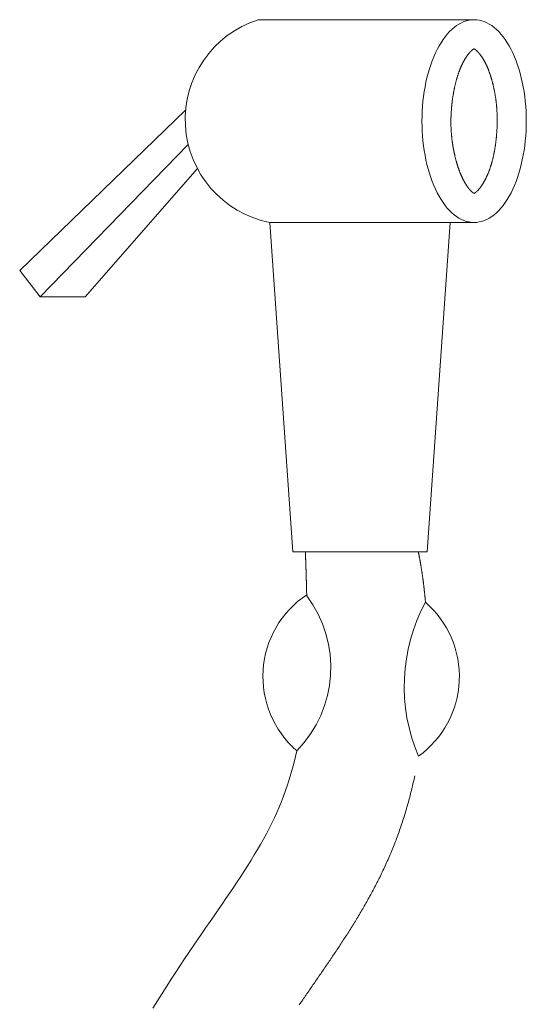
# Model space of a CAD drawing. Units: inches. Extents: x 64 to 1167, y 117 to 939.
# Tile 32 of 56: x 1044.798 to 1047.594, y 453.834 to 459.271. Entities that reach past the tile are written whole.
import ezdxf

# ---------------------------------------------------------------- set-up
doc = ezdxf.new("R2010")
doc.units = ezdxf.units.IN
doc.header["$MEASUREMENT"] = 0
doc.layers.add('A-FLOR-FIXT', color=8, linetype='Continuous', lineweight=18)

# ---------------------------------------------------------------- blocks, each defined once
blk = doc.blocks.new('A$C01277C2D')
for p, q in [((2.2872, 12.2015), (1.3927, 12.2015)), ((1.0923, 11.8276), (0.4045, 11.1621)), ((0.489, 11.0535), (1.103, 11.6838)), ((0.6759, 11.0535), (1.1406, 11.5847)), ((2.2872, 11.3612), (1.4404, 11.3612)), ((1.4404, 11.3612), (1.5365, 9.996)), ((2.0923, 9.996), (2.1874, 11.3612)), ((0.4045, 11.1621), (0.489, 11.0535)), ((0.489, 11.0535), (0.6759, 11.0535)), ((1.5365, 9.996), (2.0923, 9.996))]:
    blk.add_line(p, q)
for points in [[(2.2872, 12.2015, 0), (2.2766, 12.201, 0), (2.266, 12.1995, 0), (2.2555, 12.197, 0), (2.245, 12.1935, 0), (2.2347, 12.1889, 0), (2.2245, 12.1834, 0), (2.2144, 12.177, 0), (2.2045, 12.1695, 0), (2.1948, 12.1612, 0), (2.1853, 12.1519, 0), (2.1761, 12.1418, 0), (2.1671, 12.1307, 0), (2.1585, 12.1188, 0), (2.1501, 12.1062, 0), (2.1421, 12.0927, 0), (2.1344, 12.0785, 0), (2.1271, 12.0635, 0), (2.1201, 12.0479, 0), (2.1136, 12.0317, 0), (2.1075, 12.0148, 0), (2.1018, 11.9974, 0), (2.0966, 11.9794, 0), (2.0918, 11.961, 0), (2.0875, 11.9422, 0), (2.0837, 11.9229, 0), (2.0804, 11.9033, 0), (2.0776, 11.8835, 0), (2.0752, 11.8633, 0), (2.0734, 11.843, 0), (2.0721, 11.8226, 0), (2.0713, 11.802, 0), (2.0711, 11.7814, 0), (2.0713, 11.7608, 0), (2.0721, 11.7402, 0), (2.0734, 11.7197, 0), (2.0752, 11.6994, 0), (2.0776, 11.6793, 0), (2.0804, 11.6594, 0), (2.0837, 11.6398, 0), (2.0875, 11.6206, 0), (2.0918, 11.6017, 0), (2.0966, 11.5833, 0), (2.1018, 11.5654, 0), (2.1075, 11.548, 0), (2.1136, 11.5311, 0), (2.1201, 11.5148, 0), (2.1271, 11.4992, 0), (2.1344, 11.4843, 0), (2.1421, 11.4701, 0), (2.1501, 11.4566, 0), (2.1585, 11.4439, 0), (2.1671, 11.432, 0), (2.1761, 11.421, 0), (2.1853, 11.4108, 0), (2.1948, 11.4016, 0), (2.2045, 11.3932, 0), (2.2144, 11.3858, 0), (2.2245, 11.3793, 0), (2.2347, 11.3738, 0), (2.245, 11.3693, 0), (2.2555, 11.3658, 0), (2.266, 11.3633, 0), (2.2766, 11.3617, 0), (2.2872, 11.3612, 0), (2.2978, 11.3617, 0), (2.3084, 11.3633, 0), (2.3189, 11.3658, 0), (2.3294, 11.3693, 0), (2.3397, 11.3738, 0), (2.35, 11.3793, 0), (2.36, 11.3858, 0), (2.3699, 11.3932, 0), (2.3796, 11.4016, 0), (2.3891, 11.4108, 0), (2.3983, 11.421, 0), (2.4073, 11.432, 0), (2.416, 11.4439, 0), (2.4243, 11.4566, 0), (2.4324, 11.4701, 0), (2.44, 11.4843, 0), (2.4474, 11.4992, 0), (2.4543, 11.5148, 0), (2.4608, 11.5311, 0), (2.4669, 11.548, 0), (2.4726, 11.5654, 0), (2.4778, 11.5833, 0), (2.4826, 11.6017, 0), (2.4869, 11.6206, 0), (2.4907, 11.6398, 0), (2.494, 11.6594, 0), (2.4969, 11.6793, 0), (2.4992, 11.6994, 0), (2.501, 11.7197, 0), (2.5023, 11.7402, 0), (2.5031, 11.7608, 0), (2.5034, 11.7814, 0), (2.5031, 11.802, 0), (2.5023, 11.8226, 0), (2.501, 11.843, 0), (2.4992, 11.8633, 0), (2.4969, 11.8835, 0), (2.494, 11.9033, 0), (2.4907, 11.9229, 0), (2.4869, 11.9422, 0), (2.4826, 11.961, 0), (2.4778, 11.9794, 0), (2.4726, 11.9974, 0), (2.4669, 12.0148, 0), (2.4608, 12.0317, 0), (2.4543, 12.0479, 0), (2.4474, 12.0635, 0), (2.44, 12.0785, 0), (2.4324, 12.0927, 0), (2.4243, 12.1062, 0), (2.416, 12.1188, 0), (2.4073, 12.1307, 0), (2.3983, 12.1418, 0), (2.3891, 12.1519, 0), (2.3796, 12.1612, 0), (2.3699, 12.1695, 0), (2.36, 12.177, 0), (2.35, 12.1834, 0), (2.3397, 12.1889, 0), (2.3294, 12.1935, 0), (2.3189, 12.197, 0), (2.3084, 12.1995, 0), (2.2978, 12.201, 0), (2.2872, 12.2015, 0)], [(2.2871, 12.0812, 0), (2.2869, 12.0811, 0), (2.2868, 12.081, 0), (2.2866, 12.0809, 0), (2.2864, 12.0808, 0), (2.2861, 12.0807, 0), (2.2859, 12.0805, 0), (2.2857, 12.0804, 0), (2.2854, 12.0802, 0), (2.2851, 12.08, 0), (2.2849, 12.0799, 0), (2.2846, 12.0797, 0), (2.2843, 12.0795, 0), (2.284, 12.0793, 0), (2.2836, 12.079, 0), (2.2833, 12.0788, 0), (2.283, 12.0785, 0), (2.2826, 12.0783, 0), (2.2822, 12.078, 0), (2.2819, 12.0777, 0), (2.2815, 12.0774, 0), (2.2811, 12.0771, 0), (2.2807, 12.0768, 0), (2.2803, 12.0765, 0), (2.2799, 12.0761, 0), (2.2794, 12.0758, 0), (2.279, 12.0754, 0), (2.2786, 12.075, 0), (2.2781, 12.0746, 0), (2.2776, 12.0742, 0), (2.2772, 12.0738, 0), (2.2767, 12.0734, 0), (2.2762, 12.073, 0), (2.2757, 12.0725, 0), (2.2752, 12.072, 0), (2.2747, 12.0715, 0), (2.2742, 12.071, 0), (2.2737, 12.0705, 0), (2.2731, 12.07, 0), (2.2726, 12.0695, 0), (2.2721, 12.0689, 0), (2.2715, 12.0684, 0), (2.271, 12.0678, 0), (2.2704, 12.0672, 0), (2.2698, 12.0666, 0), (2.2693, 12.0659, 0), (2.2687, 12.0653, 0), (2.2681, 12.0647, 0), (2.2675, 12.064, 0), (2.267, 12.0633, 0), (2.2664, 12.0626, 0), (2.2658, 12.0619, 0), (2.2652, 12.0612, 0), (2.2645, 12.0604, 0), (2.2639, 12.0597, 0), (2.2633, 12.0589, 0), (2.2627, 12.0581, 0), (2.2621, 12.0573, 0), (2.2615, 12.0565, 0), (2.2608, 12.0557, 0), (2.2602, 12.0548, 0), (2.2596, 12.054, 0), (2.2589, 12.0531, 0), (2.2583, 12.0522, 0), (2.2577, 12.0513, 0), (2.257, 12.0504, 0), (2.2564, 12.0494, 0), (2.2557, 12.0485, 0), (2.2551, 12.0475, 0), (2.2545, 12.0466, 0), (2.2538, 12.0456, 0), (2.2532, 12.0446, 0), (2.2525, 12.0436, 0), (2.2519, 12.0426, 0), (2.2512, 12.0415, 0), (2.2506, 12.0405, 0), (2.25, 12.0394, 0), (2.2493, 12.0384, 0), (2.2487, 12.0373, 0), (2.248, 12.0362, 0), (2.2474, 12.0351, 0), (2.2467, 12.0339, 0), (2.2461, 12.0328, 0), (2.2454, 12.0317, 0), (2.2448, 12.0305, 0), (2.2441, 12.0293, 0), (2.2435, 12.0281, 0), (2.2428, 12.0269, 0), (2.2422, 12.0257, 0), (2.2416, 12.0245, 0), (2.2409, 12.0232, 0), (2.2403, 12.022, 0), (2.2396, 12.0207, 0), (2.239, 12.0195, 0), (2.2384, 12.0182, 0), (2.2377, 12.0169, 0), (2.2371, 12.0155, 0), (2.2365, 12.0142, 0), (2.2358, 12.0129, 0), (2.2352, 12.0115, 0), (2.2346, 12.0102, 0), (2.234, 12.0088, 0), (2.2333, 12.0074, 0), (2.2327, 12.006, 0), (2.2321, 12.0046, 0), (2.2315, 12.0032, 0), (2.2309, 12.0017, 0), (2.2303, 12.0003, 0), (2.2297, 11.9988, 0), (2.2291, 11.9974, 0), (2.2285, 11.9959, 0), (2.2279, 11.9944, 0), (2.2273, 11.9929, 0), (2.2267, 11.9913, 0), (2.2261, 11.9898, 0), (2.2255, 11.9883, 0), (2.225, 11.9867, 0), (2.2244, 11.9851, 0), (2.2238, 11.9836, 0), (2.2233, 11.982, 0), (2.2227, 11.9804, 0), (2.2221, 11.9788, 0), (2.2216, 11.9771, 0), (2.221, 11.9755, 0), (2.2205, 11.9739, 0), (2.22, 11.9722, 0), (2.2194, 11.9706, 0), (2.2189, 11.9689, 0), (2.2184, 11.9672, 0), (2.2178, 11.9655, 0), (2.2173, 11.9638, 0), (2.2168, 11.9621, 0), (2.2163, 11.9604, 0), (2.2158, 11.9586, 0), (2.2153, 11.9569, 0), (2.2148, 11.9551, 0), (2.2143, 11.9534, 0), (2.2138, 11.9516, 0), (2.2133, 11.9498, 0), (2.2128, 11.948, 0), (2.2123, 11.9462, 0), (2.2119, 11.9444, 0), (2.2114, 11.9426, 0), (2.2109, 11.9408, 0), (2.2105, 11.939, 0), (2.21, 11.9371, 0), (2.2096, 11.9353, 0), (2.2091, 11.9334, 0), (2.2087, 11.9316, 0), (2.2082, 11.9297, 0), (2.2078, 11.9278, 0), (2.2074, 11.9259, 0), (2.2069, 11.924, 0), (2.2065, 11.9221, 0), (2.2061, 11.9202, 0), (2.2057, 11.9183, 0), (2.2053, 11.9164, 0), (2.2049, 11.9145, 0), (2.2045, 11.9125, 0), (2.2041, 11.9106, 0), (2.2037, 11.9087, 0), (2.2034, 11.9067, 0), (2.203, 11.9047, 0), (2.2026, 11.9028, 0), (2.2023, 11.9008, 0), (2.2019, 11.8988, 0), (2.2016, 11.8968, 0), (2.2012, 11.8949, 0), (2.2009, 11.8929, 0), (2.2005, 11.8909, 0), (2.2002, 11.8889, 0), (2.1999, 11.8868, 0), (2.1996, 11.8848, 0), (2.1992, 11.8828, 0), (2.1989, 11.8808, 0), (2.1986, 11.8788, 0), (2.1983, 11.8767, 0), (2.198, 11.8747, 0), (2.1978, 11.8726, 0), (2.1975, 11.8706, 0), (2.1972, 11.8685, 0), (2.1969, 11.8665, 0), (2.1967, 11.8644, 0), (2.1964, 11.8623, 0), (2.1961, 11.8603, 0), (2.1959, 11.8582, 0), (2.1957, 11.8561, 0), (2.1954, 11.854, 0), (2.1952, 11.852, 0), (2.195, 11.8499, 0), (2.1947, 11.8478, 0), (2.1945, 11.8457, 0), (2.1943, 11.8436, 0), (2.1941, 11.8415, 0), (2.1939, 11.8394, 0), (2.1938, 11.8373, 0), (2.1936, 11.8352, 0), (2.1934, 11.8331, 0), (2.1932, 11.831, 0), (2.1931, 11.8289, 0), (2.1929, 11.8268, 0), (2.1928, 11.8246, 0), (2.1926, 11.8225, 0), (2.1925, 11.8204, 0), (2.1923, 11.8183, 0), (2.1922, 11.8162, 0), (2.1921, 11.814, 0), (2.192, 11.8119, 0), (2.1919, 11.8098, 0), (2.1918, 11.8077, 0), (2.1917, 11.8055, 0), (2.1916, 11.8034, 0), (2.1915, 11.8013, 0), (2.1915, 11.7992, 0), (2.1914, 11.797, 0), (2.1913, 11.7949, 0), (2.1913, 11.7928, 0), (2.1912, 11.7906, 0), (2.1912, 11.7885, 0), (2.1912, 11.7864, 0), (2.1911, 11.7842, 0), (2.1911, 11.7821, 0), (2.1911, 11.78, 0), (2.1911, 11.7779, 0), (2.1911, 11.7757, 0), (2.1911, 11.7736, 0), (2.1911, 11.7715, 0), (2.1912, 11.7694, 0), (2.1912, 11.7672, 0), (2.1912, 11.7651, 0), (2.1913, 11.763, 0), (2.1913, 11.7609, 0), (2.1914, 11.7588, 0), (2.1915, 11.7566, 0), (2.1915, 11.7545, 0), (2.1916, 11.7524, 0), (2.1917, 11.7503, 0), (2.1918, 11.7482, 0), (2.1919, 11.7461, 0), (2.192, 11.744, 0), (2.1922, 11.7419, 0), (2.1923, 11.7398, 0), (2.1924, 11.7376, 0), (2.1926, 11.7355, 0), (2.1927, 11.7335, 0), (2.1929, 11.7314, 0), (2.193, 11.7293, 0), (2.1932, 11.7272, 0), (2.1934, 11.7251, 0), (2.1936, 11.723, 0), (2.1938, 11.7209, 0), (2.194, 11.7188, 0), (2.1942, 11.7168, 0), (2.1944, 11.7147, 0), (2.1946, 11.7126, 0), (2.1948, 11.7106, 0), (2.1951, 11.7085, 0), (2.1953, 11.7064, 0), (2.1955, 11.7044, 0), (2.1958, 11.7023, 0), (2.1961, 11.7003, 0), (2.1963, 11.6982, 0), (2.1966, 11.6962, 0), (2.1969, 11.6941, 0), (2.1972, 11.6921, 0), (2.1974, 11.6901, 0), (2.1977, 11.6881, 0), (2.198, 11.686, 0), (2.1984, 11.684, 0), (2.1987, 11.682, 0), (2.199, 11.68, 0), (2.1993, 11.678, 0), (2.1996, 11.676, 0), (2.2, 11.674, 0), (2.2003, 11.672, 0), (2.2007, 11.67, 0), (2.201, 11.6681, 0), (2.2014, 11.6661, 0), (2.2018, 11.6641, 0), (2.2021, 11.6622, 0), (2.2025, 11.6602, 0), (2.2029, 11.6583, 0), (2.2033, 11.6563, 0), (2.2037, 11.6544, 0), (2.2041, 11.6525, 0), (2.2045, 11.6505, 0), (2.2049, 11.6486, 0), (2.2053, 11.6467, 0), (2.2057, 11.6448, 0), (2.2061, 11.6429, 0), (2.2066, 11.641, 0), (2.207, 11.6391, 0), (2.2074, 11.6372, 0), (2.2079, 11.6354, 0), (2.2083, 11.6335, 0), (2.2088, 11.6316, 0), (2.2092, 11.6298, 0), (2.2097, 11.6279, 0), (2.2102, 11.6261, 0), (2.2106, 11.6243, 0), (2.2111, 11.6224, 0), (2.2116, 11.6206, 0), (2.2121, 11.6188, 0), (2.2126, 11.617, 0), (2.2131, 11.6152, 0), (2.2136, 11.6135, 0), (2.2141, 11.6117, 0), (2.2146, 11.6099, 0), (2.2151, 11.6081, 0), (2.2156, 11.6064, 0), (2.2161, 11.6047, 0), (2.2166, 11.6029, 0), (2.2172, 11.6012, 0), (2.2177, 11.5995, 0), (2.2182, 11.5978, 0), (2.2188, 11.5961, 0), (2.2193, 11.5944, 0), (2.2199, 11.5927, 0), (2.2204, 11.591, 0), (2.221, 11.5894, 0), (2.2215, 11.5877, 0), (2.2221, 11.5861, 0), (2.2226, 11.5844, 0), (2.2232, 11.5828, 0), (2.2238, 11.5812, 0), (2.2243, 11.5796, 0), (2.2249, 11.578, 0), (2.2255, 11.5764, 0), (2.2261, 11.5749, 0), (2.2267, 11.5733, 0), (2.2273, 11.5717, 0), (2.2279, 11.5702, 0), (2.2285, 11.5687, 0), (2.2291, 11.5671, 0), (2.2297, 11.5656, 0), (2.2303, 11.5641, 0), (2.2309, 11.5626, 0), (2.2315, 11.5612, 0), (2.2321, 11.5597, 0), (2.2327, 11.5582, 0), (2.2333, 11.5568, 0), (2.234, 11.5554, 0), (2.2346, 11.554, 0), (2.2352, 11.5526, 0), (2.2358, 11.5512, 0), (2.2365, 11.5498, 0), (2.2371, 11.5485, 0), (2.2377, 11.5471, 0), (2.2384, 11.5458, 0), (2.239, 11.5445, 0), (2.2396, 11.5432, 0), (2.2403, 11.5419, 0), (2.2409, 11.5406, 0), (2.2416, 11.5394, 0), (2.2422, 11.5381, 0), (2.2428, 11.5369, 0), (2.2435, 11.5357, 0), (2.2441, 11.5345, 0), (2.2448, 11.5333, 0), (2.2454, 11.5321, 0), (2.246, 11.531, 0), (2.2467, 11.5298, 0), (2.2473, 11.5287, 0), (2.248, 11.5276, 0), (2.2486, 11.5265, 0), (2.2493, 11.5254, 0), (2.2499, 11.5243, 0), (2.2505, 11.5233, 0), (2.2512, 11.5222, 0), (2.2518, 11.5212, 0), (2.2525, 11.5202, 0), (2.2531, 11.5191, 0), (2.2537, 11.5182, 0), (2.2544, 11.5172, 0), (2.255, 11.5162, 0), (2.2556, 11.5153, 0), (2.2562, 11.5143, 0), (2.2569, 11.5134, 0), (2.2575, 11.5125, 0), (2.2581, 11.5116, 0), (2.2587, 11.5107, 0), (2.2593, 11.5098, 0), (2.2599, 11.509, 0), (2.2605, 11.5081, 0), (2.2612, 11.5073, 0), (2.2618, 11.5065, 0), (2.2624, 11.5057, 0), (2.2629, 11.5049, 0), (2.2635, 11.5041, 0), (2.2641, 11.5034, 0), (2.2647, 11.5026, 0), (2.2653, 11.5019, 0), (2.2659, 11.5012, 0), (2.2664, 11.5005, 0), (2.267, 11.4998, 0), (2.2676, 11.4991, 0), (2.2681, 11.4985, 0), (2.2687, 11.4978, 0), (2.2692, 11.4972, 0), (2.2698, 11.4966, 0), (2.2703, 11.4959, 0), (2.2708, 11.4953, 0), (2.2714, 11.4948, 0), (2.2719, 11.4942, 0), (2.2724, 11.4936, 0), (2.2729, 11.4931, 0), (2.2734, 11.4926, 0), (2.2739, 11.4921, 0), (2.2744, 11.4916, 0), (2.2749, 11.4911, 0), (2.2754, 11.4906, 0), (2.2759, 11.4901, 0), (2.2763, 11.4897, 0), (2.2768, 11.4892, 0), (2.2772, 11.4888, 0), (2.2777, 11.4884, 0), (2.2781, 11.488, 0), (2.2786, 11.4876, 0), (2.279, 11.4873, 0), (2.2794, 11.4869, 0), (2.2798, 11.4866, 0), (2.2802, 11.4863, 0), (2.2806, 11.4859, 0), (2.281, 11.4856, 0), (2.2814, 11.4854, 0), (2.2817, 11.4851, 0), (2.2821, 11.4848, 0), (2.2825, 11.4846, 0), (2.2828, 11.4843, 0), (2.2831, 11.4841, 0), (2.2835, 11.4839, 0), (2.2838, 11.4837, 0), (2.2841, 11.4835, 0), (2.2844, 11.4833, 0), (2.2847, 11.4831, 0), (2.285, 11.4829, 0), (2.2852, 11.4828, 0), (2.2855, 11.4826, 0), (2.2858, 11.4825, 0), (2.286, 11.4823, 0), (2.2862, 11.4822, 0), (2.2865, 11.4821, 0), (2.2867, 11.482, 0), (2.2869, 11.4818, 0), (2.2871, 11.4818, 0), (2.2873, 11.4817, 0), (2.2875, 11.4816, 0), (2.2876, 11.4815, 0)], [(2.2876, 11.4815, 0), (2.2878, 11.4816, 0), (2.2881, 11.4817, 0), (2.2883, 11.4819, 0), (2.2886, 11.482, 0), (2.2888, 11.4822, 0), (2.2891, 11.4824, 0), (2.2894, 11.4826, 0), (2.2898, 11.4828, 0), (2.2901, 11.4831, 0), (2.2904, 11.4833, 0), (2.2908, 11.4836, 0), (2.2912, 11.4838, 0), (2.2916, 11.4841, 0), (2.292, 11.4845, 0), (2.2924, 11.4848, 0), (2.2929, 11.4851, 0), (2.2933, 11.4855, 0), (2.2938, 11.4859, 0), (2.2943, 11.4863, 0), (2.2948, 11.4867, 0), (2.2953, 11.4871, 0), (2.2958, 11.4875, 0), (2.2963, 11.488, 0), (2.2969, 11.4885, 0), (2.2974, 11.489, 0), (2.298, 11.4895, 0), (2.2985, 11.49, 0), (2.2991, 11.4906, 0), (2.2997, 11.4911, 0), (2.3003, 11.4917, 0), (2.3009, 11.4923, 0), (2.3015, 11.493, 0), (2.3021, 11.4936, 0), (2.3028, 11.4943, 0), (2.3034, 11.4949, 0), (2.3041, 11.4956, 0), (2.3047, 11.4963, 0), (2.3054, 11.4971, 0), (2.306, 11.4978, 0), (2.3067, 11.4986, 0), (2.3074, 11.4994, 0), (2.3081, 11.5002, 0), (2.3088, 11.501, 0), (2.3095, 11.5019, 0), (2.3102, 11.5027, 0), (2.3109, 11.5036, 0), (2.3116, 11.5045, 0), (2.3123, 11.5055, 0), (2.313, 11.5064, 0), (2.3138, 11.5074, 0), (2.3145, 11.5084, 0), (2.3152, 11.5094, 0), (2.3159, 11.5104, 0), (2.3167, 11.5115, 0), (2.3174, 11.5125, 0), (2.3181, 11.5136, 0), (2.3189, 11.5147, 0), (2.3196, 11.5159, 0), (2.3204, 11.517, 0), (2.3211, 11.5182, 0), (2.3219, 11.5193, 0), (2.3226, 11.5205, 0), (2.3234, 11.5218, 0), (2.3241, 11.523, 0), (2.3249, 11.5243, 0), (2.3256, 11.5255, 0), (2.3264, 11.5268, 0), (2.3271, 11.5281, 0), (2.3279, 11.5294, 0), (2.3287, 11.5308, 0), (2.3294, 11.5321, 0), (2.3302, 11.5335, 0), (2.3309, 11.5349, 0), (2.3317, 11.5363, 0), (2.3324, 11.5377, 0), (2.3332, 11.5392, 0), (2.3339, 11.5406, 0), (2.3347, 11.5421, 0), (2.3354, 11.5436, 0), (2.3362, 11.5451, 0), (2.3369, 11.5466, 0), (2.3377, 11.5481, 0), (2.3384, 11.5497, 0), (2.3391, 11.5513, 0), (2.3399, 11.5528, 0), (2.3406, 11.5544, 0), (2.3413, 11.556, 0), (2.342, 11.5577, 0), (2.3428, 11.5593, 0), (2.3435, 11.561, 0), (2.3442, 11.5626, 0), (2.3449, 11.5643, 0), (2.3456, 11.566, 0), (2.3463, 11.5677, 0), (2.347, 11.5694, 0), (2.3477, 11.5712, 0), (2.3484, 11.5729, 0), (2.3491, 11.5747, 0), (2.3497, 11.5765, 0), (2.3504, 11.5783, 0), (2.3511, 11.5801, 0), (2.3517, 11.5819, 0), (2.3524, 11.5837, 0), (2.353, 11.5856, 0), (2.3537, 11.5874, 0), (2.3543, 11.5893, 0), (2.3549, 11.5912, 0), (2.3556, 11.5931, 0), (2.3562, 11.595, 0), (2.3568, 11.5969, 0), (2.3574, 11.5989, 0), (2.358, 11.6008, 0), (2.3586, 11.6028, 0), (2.3591, 11.6048, 0), (2.3597, 11.6068, 0), (2.3603, 11.6088, 0), (2.3609, 11.6108, 0), (2.3614, 11.6128, 0), (2.362, 11.6148, 0), (2.3625, 11.6169, 0), (2.363, 11.6189, 0), (2.3636, 11.621, 0), (2.3641, 11.6231, 0), (2.3646, 11.6252, 0), (2.3651, 11.6273, 0), (2.3656, 11.6294, 0), (2.3661, 11.6315, 0), (2.3666, 11.6337, 0), (2.3671, 11.6358, 0), (2.3676, 11.638, 0), (2.3681, 11.6402, 0), (2.3685, 11.6423, 0), (2.369, 11.6445, 0), (2.3694, 11.6467, 0), (2.3699, 11.6489, 0), (2.3703, 11.6511, 0), (2.3707, 11.6534, 0), (2.3712, 11.6556, 0), (2.3716, 11.6578, 0), (2.372, 11.6601, 0), (2.3724, 11.6623, 0), (2.3728, 11.6646, 0), (2.3732, 11.6669, 0), (2.3735, 11.6692, 0), (2.3739, 11.6714, 0), (2.3743, 11.6737, 0), (2.3746, 11.676, 0), (2.375, 11.6783, 0), (2.3753, 11.6807, 0), (2.3757, 11.683, 0), (2.376, 11.6853, 0), (2.3763, 11.6877, 0), (2.3766, 11.69, 0), (2.3769, 11.6924, 0), (2.3772, 11.6947, 0), (2.3775, 11.6971, 0), (2.3778, 11.6994, 0), (2.3781, 11.7018, 0), (2.3783, 11.7042, 0), (2.3786, 11.7066, 0), (2.3789, 11.709, 0), (2.3791, 11.7113, 0), (2.3793, 11.7137, 0), (2.3796, 11.7161, 0), (2.3798, 11.7186, 0), (2.38, 11.721, 0), (2.3802, 11.7234, 0), (2.3804, 11.7258, 0), (2.3806, 11.7282, 0), (2.3808, 11.7306, 0), (2.381, 11.7331, 0), (2.3811, 11.7355, 0), (2.3813, 11.7379, 0), (2.3814, 11.7404, 0), (2.3816, 11.7428, 0), (2.3817, 11.7453, 0), (2.3819, 11.7477, 0), (2.382, 11.7502, 0), (2.3821, 11.7526, 0), (2.3822, 11.7551, 0), (2.3823, 11.7575, 0), (2.3824, 11.76, 0), (2.3824, 11.7624, 0), (2.3825, 11.7649, 0), (2.3826, 11.7674, 0), (2.3826, 11.7698, 0), (2.3827, 11.7723, 0), (2.3827, 11.7747, 0), (2.3827, 11.7772, 0), (2.3828, 11.7797, 0), (2.3828, 11.7821, 0), (2.3828, 11.7846, 0), (2.3828, 11.7871, 0), (2.3828, 11.7895, 0), (2.3827, 11.792, 0), (2.3827, 11.7945, 0), (2.3827, 11.7969, 0), (2.3826, 11.7994, 0), (2.3826, 11.8018, 0), (2.3825, 11.8043, 0), (2.3824, 11.8068, 0), (2.3824, 11.8092, 0), (2.3823, 11.8117, 0), (2.3822, 11.8141, 0), (2.3821, 11.8166, 0), (2.3819, 11.819, 0), (2.3818, 11.8215, 0), (2.3817, 11.8239, 0), (2.3815, 11.8263, 0), (2.3814, 11.8288, 0), (2.3812, 11.8312, 0), (2.3811, 11.8336, 0), (2.3809, 11.8361, 0), (2.3807, 11.8385, 0), (2.3805, 11.8409, 0), (2.3803, 11.8433, 0), (2.3801, 11.8458, 0), (2.3798, 11.8482, 0), (2.3796, 11.8506, 0), (2.3794, 11.853, 0), (2.3791, 11.8554, 0), (2.3789, 11.8578, 0), (2.3786, 11.8601, 0), (2.3783, 11.8625, 0), (2.378, 11.8649, 0), (2.3777, 11.8673, 0), (2.3774, 11.8696, 0), (2.3771, 11.872, 0), (2.3768, 11.8743, 0), (2.3765, 11.8767, 0), (2.3761, 11.879, 0), (2.3758, 11.8814, 0), (2.3754, 11.8837, 0), (2.375, 11.886, 0), (2.3746, 11.8883, 0), (2.3743, 11.8906, 0), (2.3739, 11.8929, 0), (2.3735, 11.8952, 0), (2.3731, 11.8975, 0), (2.3727, 11.8998, 0), (2.3722, 11.902, 0), (2.3718, 11.9043, 0), (2.3714, 11.9065, 0), (2.3709, 11.9088, 0), (2.3705, 11.911, 0), (2.37, 11.9132, 0), (2.3695, 11.9154, 0), (2.3691, 11.9176, 0), (2.3686, 11.9198, 0), (2.3681, 11.922, 0), (2.3676, 11.9241, 0), (2.3671, 11.9263, 0), (2.3666, 11.9285, 0), (2.3661, 11.9306, 0), (2.3656, 11.9327, 0), (2.3651, 11.9349, 0), (2.3645, 11.937, 0), (2.364, 11.9391, 0), (2.3634, 11.9412, 0), (2.3629, 11.9432, 0), (2.3624, 11.9453, 0), (2.3618, 11.9474, 0), (2.3612, 11.9494, 0), (2.3607, 11.9514, 0), (2.3601, 11.9535, 0), (2.3595, 11.9555, 0), (2.3589, 11.9575, 0), (2.3583, 11.9594, 0), (2.3577, 11.9614, 0), (2.3571, 11.9634, 0), (2.3565, 11.9653, 0), (2.3559, 11.9673, 0), (2.3553, 11.9692, 0), (2.3546, 11.9711, 0), (2.354, 11.973, 0), (2.3534, 11.9749, 0), (2.3527, 11.9768, 0), (2.3521, 11.9786, 0), (2.3514, 11.9805, 0), (2.3508, 11.9823, 0), (2.3501, 11.9841, 0), (2.3495, 11.9859, 0), (2.3488, 11.9877, 0), (2.3481, 11.9895, 0), (2.3475, 11.9912, 0), (2.3468, 11.993, 0), (2.3461, 11.9947, 0), (2.3454, 11.9964, 0), (2.3448, 11.9981, 0), (2.3441, 11.9998, 0), (2.3434, 12.0015, 0), (2.3427, 12.0032, 0), (2.342, 12.0048, 0), (2.3413, 12.0064, 0), (2.3406, 12.008, 0), (2.3399, 12.0096, 0), (2.3392, 12.0112, 0), (2.3384, 12.0128, 0), (2.3377, 12.0143, 0), (2.337, 12.0159, 0), (2.3363, 12.0174, 0), (2.3356, 12.0189, 0), (2.3348, 12.0203, 0), (2.3341, 12.0218, 0), (2.3334, 12.0233, 0), (2.3326, 12.0247, 0), (2.3319, 12.0261, 0), (2.3312, 12.0275, 0), (2.3304, 12.0289, 0), (2.3297, 12.0302, 0), (2.3289, 12.0316, 0), (2.3282, 12.0329, 0), (2.3274, 12.0342, 0), (2.3267, 12.0355, 0), (2.326, 12.0368, 0), (2.3252, 12.038, 0), (2.3245, 12.0393, 0), (2.3237, 12.0405, 0), (2.323, 12.0417, 0), (2.3222, 12.0429, 0), (2.3215, 12.044, 0), (2.3207, 12.0451, 0), (2.32, 12.0463, 0), (2.3192, 12.0474, 0), (2.3185, 12.0484, 0), (2.3177, 12.0495, 0), (2.317, 12.0505, 0), (2.3163, 12.0516, 0), (2.3155, 12.0526, 0), (2.3148, 12.0535, 0), (2.3141, 12.0545, 0), (2.3134, 12.0555, 0), (2.3127, 12.0564, 0), (2.312, 12.0573, 0), (2.3112, 12.0582, 0), (2.3106, 12.0591, 0), (2.3099, 12.0599, 0), (2.3092, 12.0608, 0), (2.3085, 12.0616, 0), (2.3078, 12.0624, 0), (2.3071, 12.0632, 0), (2.3065, 12.0639, 0), (2.3058, 12.0647, 0), (2.3052, 12.0654, 0), (2.3045, 12.0661, 0), (2.3039, 12.0668, 0), (2.3032, 12.0675, 0), (2.3026, 12.0682, 0), (2.302, 12.0688, 0), (2.3014, 12.0694, 0), (2.3008, 12.07, 0), (2.3002, 12.0706, 0), (2.2996, 12.0712, 0), (2.299, 12.0718, 0), (2.2985, 12.0723, 0), (2.2979, 12.0728, 0), (2.2974, 12.0733, 0), (2.2968, 12.0738, 0), (2.2963, 12.0743, 0), (2.2958, 12.0748, 0), (2.2953, 12.0752, 0), (2.2948, 12.0757, 0), (2.2943, 12.0761, 0), (2.2938, 12.0765, 0), (2.2933, 12.0769, 0), (2.2929, 12.0772, 0), (2.2924, 12.0776, 0), (2.292, 12.0779, 0), (2.2916, 12.0782, 0), (2.2912, 12.0785, 0), (2.2908, 12.0788, 0), (2.2904, 12.0791, 0), (2.29, 12.0794, 0), (2.2897, 12.0796, 0), (2.2893, 12.0799, 0), (2.289, 12.0801, 0), (2.2887, 12.0803, 0), (2.2884, 12.0805, 0), (2.2881, 12.0806, 0), (2.2878, 12.0808, 0), (2.2876, 12.0809, 0), (2.2873, 12.0811, 0), (2.2871, 12.0812, 0)], [(1.5938, 9.8141, 0), (1.5937, 9.8155, 0), (1.5937, 9.817, 0), (1.5937, 9.8184, 0), (1.5936, 9.8198, 0), (1.5936, 9.8212, 0), (1.5936, 9.8227, 0), (1.5935, 9.8241, 0), (1.5935, 9.8255, 0), (1.5934, 9.827, 0), (1.5934, 9.8284, 0), (1.5934, 9.8298, 0), (1.5934, 9.8313, 0), (1.5933, 9.8327, 0), (1.5933, 9.8341, 0), (1.5932, 9.8355, 0), (1.5932, 9.837, 0), (1.5932, 9.8384, 0), (1.5931, 9.8398, 0), (1.5931, 9.8413, 0), (1.5931, 9.8427, 0), (1.593, 9.8441, 0), (1.593, 9.8456, 0), (1.5929, 9.847, 0), (1.5929, 9.8484, 0), (1.5929, 9.8498, 0), (1.5928, 9.8513, 0), (1.5928, 9.8527, 0), (1.5927, 9.8541, 0), (1.5927, 9.8556, 0), (1.5927, 9.857, 0), (1.5926, 9.8584, 0), (1.5926, 9.8599, 0), (1.5925, 9.8613, 0), (1.5925, 9.8627, 0), (1.5925, 9.8642, 0), (1.5924, 9.8656, 0), (1.5924, 9.867, 0), (1.5923, 9.8684, 0), (1.5923, 9.8699, 0), (1.5923, 9.8713, 0), (1.5922, 9.8727, 0), (1.5922, 9.8742, 0), (1.5921, 9.8756, 0), (1.5921, 9.877, 0), (1.592, 9.8785, 0), (1.592, 9.8799, 0), (1.592, 9.8813, 0), (1.5919, 9.8828, 0), (1.5919, 9.8842, 0), (1.5918, 9.8856, 0), (1.5918, 9.8871, 0), (1.5917, 9.8885, 0), (1.5917, 9.8899, 0), (1.5917, 9.8914, 0), (1.5916, 9.8928, 0), (1.5916, 9.8942, 0), (1.5915, 9.8956, 0), (1.5915, 9.8971, 0), (1.5915, 9.8985, 0), (1.5914, 9.9, 0), (1.5914, 9.9014, 0), (1.5913, 9.9028, 0), (1.5913, 9.9042, 0), (1.5912, 9.9057, 0), (1.5912, 9.9071, 0), (1.5911, 9.9085, 0), (1.5911, 9.91, 0), (1.5911, 9.9114, 0), (1.591, 9.9129, 0), (1.591, 9.9143, 0), (1.5909, 9.9157, 0), (1.5909, 9.9171, 0), (1.5908, 9.9186, 0), (1.5908, 9.92, 0), (1.5907, 9.9215, 0), (1.5907, 9.9229, 0), (1.5906, 9.9243, 0), (1.5906, 9.9258, 0), (1.5905, 9.9272, 0), (1.5905, 9.9286, 0), (1.5904, 9.93, 0), (1.5904, 9.9315, 0), (1.5904, 9.9329, 0), (1.5903, 9.9344, 0), (1.5903, 9.9358, 0), (1.5902, 9.9372, 0), (1.5902, 9.9387, 0), (1.5901, 9.9401, 0), (1.5901, 9.9415, 0), (1.59, 9.9429, 0), (1.59, 9.9444, 0), (1.5899, 9.9458, 0), (1.5899, 9.9473, 0), (1.5898, 9.9487, 0), (1.5898, 9.9501, 0), (1.5897, 9.9515, 0), (1.5897, 9.953, 0), (1.5896, 9.9544, 0), (1.5896, 9.9558, 0), (1.5896, 9.9573, 0), (1.5895, 9.9587, 0), (1.5895, 9.9602, 0), (1.5894, 9.9616, 0), (1.5894, 9.963, 0), (1.5893, 9.9645, 0), (1.5893, 9.9659, 0), (1.5892, 9.9673, 0), (1.5892, 9.9688, 0), (1.5891, 9.9702, 0), (1.5891, 9.9716, 0), (1.589, 9.9731, 0), (1.589, 9.9745, 0), (1.5889, 9.9759, 0), (1.5889, 9.9774, 0), (1.5888, 9.9788, 0), (1.5888, 9.9802, 0), (1.5887, 9.9817, 0), (1.5887, 9.9831, 0), (1.5886, 9.9845, 0), (1.5886, 9.986, 0), (1.5885, 9.9874, 0), (1.5885, 9.9888, 0), (1.5884, 9.9903, 0), (1.5884, 9.9917, 0), (1.5883, 9.9931, 0), (1.5883, 9.9946, 0), (1.5882, 9.996, 0)], [(2.0856, 9.787, 0), (2.0854, 9.7887, 0), (2.0853, 9.7904, 0), (2.0852, 9.7922, 0), (2.085, 9.7939, 0), (2.0848, 9.7956, 0), (2.0847, 9.7973, 0), (2.0845, 9.7991, 0), (2.0844, 9.8008, 0), (2.0842, 9.8025, 0), (2.084, 9.8042, 0), (2.0839, 9.806, 0), (2.0837, 9.8077, 0), (2.0836, 9.8094, 0), (2.0834, 9.8111, 0), (2.0832, 9.8128, 0), (2.0831, 9.8145, 0), (2.0829, 9.8163, 0), (2.0827, 9.818, 0), (2.0825, 9.8197, 0), (2.0824, 9.8214, 0), (2.0822, 9.8231, 0), (2.082, 9.8248, 0), (2.0818, 9.8265, 0), (2.0817, 9.8282, 0), (2.0815, 9.8299, 0), (2.0813, 9.8316, 0), (2.0811, 9.8333, 0), (2.0809, 9.835, 0), (2.0808, 9.8367, 0), (2.0806, 9.8384, 0), (2.0804, 9.8401, 0), (2.0802, 9.8418, 0), (2.08, 9.8435, 0), (2.0798, 9.8452, 0), (2.0796, 9.8468, 0), (2.0794, 9.8485, 0), (2.0792, 9.8502, 0), (2.079, 9.8519, 0), (2.0788, 9.8536, 0), (2.0786, 9.8553, 0), (2.0784, 9.8569, 0), (2.0782, 9.8586, 0), (2.078, 9.8603, 0), (2.0778, 9.862, 0), (2.0776, 9.8636, 0), (2.0774, 9.8653, 0), (2.0772, 9.867, 0), (2.077, 9.8687, 0), (2.0768, 9.8703, 0), (2.0765, 9.872, 0), (2.0763, 9.8737, 0), (2.0761, 9.8753, 0), (2.0759, 9.877, 0), (2.0757, 9.8787, 0), (2.0755, 9.8803, 0), (2.0752, 9.882, 0), (2.075, 9.8836, 0), (2.0748, 9.8853, 0), (2.0746, 9.887, 0), (2.0743, 9.8886, 0), (2.0741, 9.8902, 0), (2.0739, 9.8919, 0), (2.0736, 9.8935, 0), (2.0734, 9.8952, 0), (2.0732, 9.8969, 0), (2.0729, 9.8985, 0), (2.0727, 9.9001, 0), (2.0725, 9.9018, 0), (2.0722, 9.9034, 0), (2.072, 9.9051, 0), (2.0718, 9.9067, 0), (2.0715, 9.9083, 0), (2.0713, 9.91, 0), (2.071, 9.9116, 0), (2.0708, 9.9132, 0), (2.0705, 9.9149, 0), (2.0703, 9.9165, 0), (2.07, 9.9181, 0), (2.0698, 9.9197, 0), (2.0695, 9.9214, 0), (2.0693, 9.923, 0), (2.069, 9.9246, 0), (2.0688, 9.9262, 0), (2.0685, 9.9278, 0), (2.0682, 9.9295, 0), (2.068, 9.9311, 0), (2.0677, 9.9327, 0), (2.0675, 9.9343, 0), (2.0672, 9.9359, 0), (2.0669, 9.9375, 0), (2.0667, 9.9391, 0), (2.0664, 9.9407, 0), (2.0661, 9.9423, 0), (2.0658, 9.944, 0), (2.0656, 9.9456, 0), (2.0653, 9.9472, 0), (2.065, 9.9488, 0), (2.0648, 9.9504, 0), (2.0645, 9.952, 0), (2.0642, 9.9535, 0), (2.0639, 9.9551, 0), (2.0636, 9.9567, 0), (2.0633, 9.9583, 0), (2.0631, 9.9599, 0), (2.0628, 9.9615, 0), (2.0625, 9.9631, 0), (2.0622, 9.9647, 0), (2.0619, 9.9662, 0), (2.0616, 9.9678, 0), (2.0613, 9.9694, 0), (2.061, 9.971, 0), (2.0607, 9.9726, 0), (2.0604, 9.9741, 0), (2.0601, 9.9757, 0), (2.0598, 9.9773, 0), (2.0596, 9.9788, 0), (2.0592, 9.9804, 0), (2.0589, 9.982, 0), (2.0586, 9.9835, 0), (2.0583, 9.9851, 0), (2.058, 9.9867, 0), (2.0577, 9.9882, 0), (2.0574, 9.9898, 0), (2.0571, 9.9914, 0), (2.0568, 9.9929, 0), (2.0565, 9.9945, 0), (2.0562, 9.996, 0)], [(0.9566, 8.1047, 0), (0.9757, 8.1358, 0), (0.9946, 8.1662, 0), (1.0135, 8.1959, 0), (1.0322, 8.2251, 0), (1.0508, 8.2536, 0), (1.0692, 8.2816, 0), (1.0875, 8.3091, 0), (1.1056, 8.336, 0), (1.1236, 8.3625, 0), (1.1413, 8.3885, 0), (1.1588, 8.414, 0), (1.1761, 8.4392, 0), (1.1932, 8.4639, 0), (1.2101, 8.4883, 0), (1.2267, 8.5124, 0), (1.243, 8.5361, 0), (1.2591, 8.5596, 0), (1.2749, 8.5828, 0), (1.2904, 8.6057, 0), (1.3056, 8.6285, 0), (1.3204, 8.651, 0), (1.335, 8.6734, 0), (1.3492, 8.6957, 0), (1.3631, 8.7178, 0), (1.3766, 8.7399, 0), (1.3897, 8.7619, 0), (1.4024, 8.7838, 0), (1.4148, 8.8058, 0), (1.4267, 8.8277, 0), (1.4382, 8.8497, 0), (1.4493, 8.8718, 0), (1.46, 8.8939, 0), (1.4702, 8.9162, 0), (1.4799, 8.9386, 0), (1.4892, 8.9612, 0), (1.4979, 8.9839, 0), (1.5063, 9.0068, 0), (1.5141, 9.0299, 0), (1.5215, 9.0532, 0), (1.5285, 9.0767, 0), (1.535, 9.1003, 0), (1.5412, 9.124, 0), (1.5469, 9.1479, 0), (1.5523, 9.172, 0)], [(1.5627, 8.1187, 0), (1.5662, 8.1239, 0), (1.5698, 8.1291, 0), (1.5734, 8.1343, 0), (1.5769, 8.1395, 0), (1.5805, 8.1446, 0), (1.584, 8.1498, 0), (1.5876, 8.155, 0), (1.5912, 8.1601, 0), (1.5947, 8.1653, 0), (1.5983, 8.1704, 0), (1.6018, 8.1756, 0), (1.6054, 8.1807, 0), (1.6089, 8.1859, 0), (1.6125, 8.191, 0), (1.616, 8.1962, 0), (1.6196, 8.2013, 0), (1.6231, 8.2065, 0), (1.6267, 8.2116, 0), (1.6302, 8.2168, 0), (1.6338, 8.2219, 0), (1.6373, 8.2271, 0), (1.6408, 8.2322, 0), (1.6444, 8.2373, 0), (1.6479, 8.2425, 0), (1.6515, 8.2476, 0), (1.655, 8.2528, 0), (1.6585, 8.2579, 0), (1.6621, 8.2631, 0), (1.6656, 8.2683, 0), (1.6692, 8.2734, 0), (1.6727, 8.2786, 0), (1.6762, 8.2838, 0), (1.6798, 8.289, 0), (1.6833, 8.2942, 0), (1.6868, 8.2994, 0), (1.6904, 8.3046, 0), (1.6939, 8.3098, 0), (1.6974, 8.315, 0), (1.701, 8.3202, 0), (1.7045, 8.3255, 0), (1.708, 8.3307, 0), (1.7116, 8.336, 0), (1.7151, 8.3412, 0), (1.7186, 8.3465, 0), (1.7221, 8.3518, 0), (1.7256, 8.357, 0), (1.7291, 8.3624, 0), (1.7327, 8.3677, 0), (1.7362, 8.373, 0), (1.7396, 8.3783, 0), (1.7431, 8.3837, 0), (1.7466, 8.389, 0), (1.7501, 8.3944, 0), (1.7536, 8.3998, 0), (1.7571, 8.4052, 0), (1.7606, 8.4106, 0), (1.764, 8.4161, 0), (1.7675, 8.4215, 0), (1.771, 8.427, 0), (1.7744, 8.4324, 0), (1.7779, 8.4379, 0), (1.7813, 8.4435, 0), (1.7848, 8.449, 0), (1.7882, 8.4545, 0), (1.7916, 8.4601, 0), (1.7951, 8.4657, 0), (1.7985, 8.4713, 0), (1.8019, 8.4769, 0), (1.8053, 8.4825, 0), (1.8087, 8.4882, 0), (1.8121, 8.4938, 0), (1.8155, 8.4995, 0), (1.8189, 8.5053, 0), (1.8222, 8.511, 0), (1.8256, 8.5167, 0), (1.829, 8.5225, 0), (1.8323, 8.5283, 0), (1.8356, 8.5341, 0), (1.839, 8.54, 0), (1.8423, 8.5458, 0), (1.8456, 8.5517, 0), (1.8489, 8.5577, 0), (1.8522, 8.5636, 0), (1.8555, 8.5696, 0), (1.8588, 8.5755, 0), (1.862, 8.5816, 0), (1.8653, 8.5876, 0), (1.8685, 8.5937, 0), (1.8718, 8.5999, 0), (1.875, 8.606, 0), (1.8782, 8.6122, 0), (1.8814, 8.6184, 0), (1.8846, 8.6247, 0), (1.8878, 8.631, 0), (1.891, 8.6372, 0), (1.8941, 8.6436, 0), (1.8973, 8.6499, 0), (1.9004, 8.6563, 0), (1.9035, 8.6627, 0), (1.9065, 8.6692, 0), (1.9096, 8.6756, 0), (1.9127, 8.6821, 0), (1.9157, 8.6886, 0), (1.9187, 8.6951, 0), (1.9217, 8.7017, 0), (1.9246, 8.7082, 0), (1.9276, 8.7148, 0), (1.9305, 8.7214, 0), (1.9334, 8.7281, 0), (1.9363, 8.7347, 0), (1.9391, 8.7414, 0), (1.942, 8.748, 0), (1.9448, 8.7547, 0), (1.9475, 8.7614, 0), (1.9503, 8.7682, 0), (1.953, 8.7749, 0), (1.9557, 8.7816, 0), (1.9584, 8.7884, 0), (1.961, 8.7952, 0), (1.9636, 8.8019, 0), (1.9662, 8.8087, 0), (1.9687, 8.8155, 0), (1.9712, 8.8224, 0), (1.9737, 8.8292, 0), (1.9762, 8.836, 0), (1.9786, 8.8429, 0), (1.981, 8.8497, 0), (1.9833, 8.8565, 0), (1.9856, 8.8634, 0), (1.9879, 8.8702, 0), (1.9902, 8.8771, 0), (1.9924, 8.8839, 0), (1.9946, 8.8908, 0), (1.9968, 8.8976, 0), (1.9989, 8.9044, 0), (2.001, 8.9113, 0), (2.003, 8.9181, 0), (2.0051, 8.9249, 0), (2.0071, 8.9318, 0), (2.0091, 8.9386, 0), (2.011, 8.9454, 0), (2.0129, 8.9522, 0), (2.0148, 8.9591, 0), (2.0167, 8.9659, 0), (2.0185, 8.9727, 0), (2.0203, 8.9795, 0), (2.0221, 8.9863, 0), (2.0238, 8.9931, 0), (2.0255, 8.9999, 0), (2.0272, 9.0067, 0), (2.0289, 9.0135, 0), (2.0305, 9.0203, 0), (2.0321, 9.027, 0), (2.0337, 9.0338, 0), (2.0353, 9.0406, 0), (2.0368, 9.0474, 0), (2.0383, 9.0541, 0), (2.0398, 9.0609, 0), (2.0412, 9.0676, 0)]]:
    blk.add_polyline3d(points)
for centre, radius, start, end in [((1.525, 11.7875), 0.4346, 107.72, 258.7669), ((1.819, 9.4794), 0.407, 123.6217, 229.0465), ((1.201, 9.5171), 0.4924, 315.509, 37.0937), ((2.7306, 9.4385), 0.7332, 151.6203, 203.2399), ((1.819, 9.4794), 0.407, 305.7764, 49.0838)]:
    blk.add_arc(centre, radius, start, end)

msp = doc.modelspace()

# ---------------------------------------------------------------- block references
at = {"layer": 'A-FLOR-FIXT', "xscale": 1.33257137012807, "yscale": 1.33257137012807, "zscale": 1.33257137012807}
msp.add_blockref('A$C01277C2D', (1044.2585, 443.012), dxfattribs=at)

doc.saveas('drawing.dxf')
